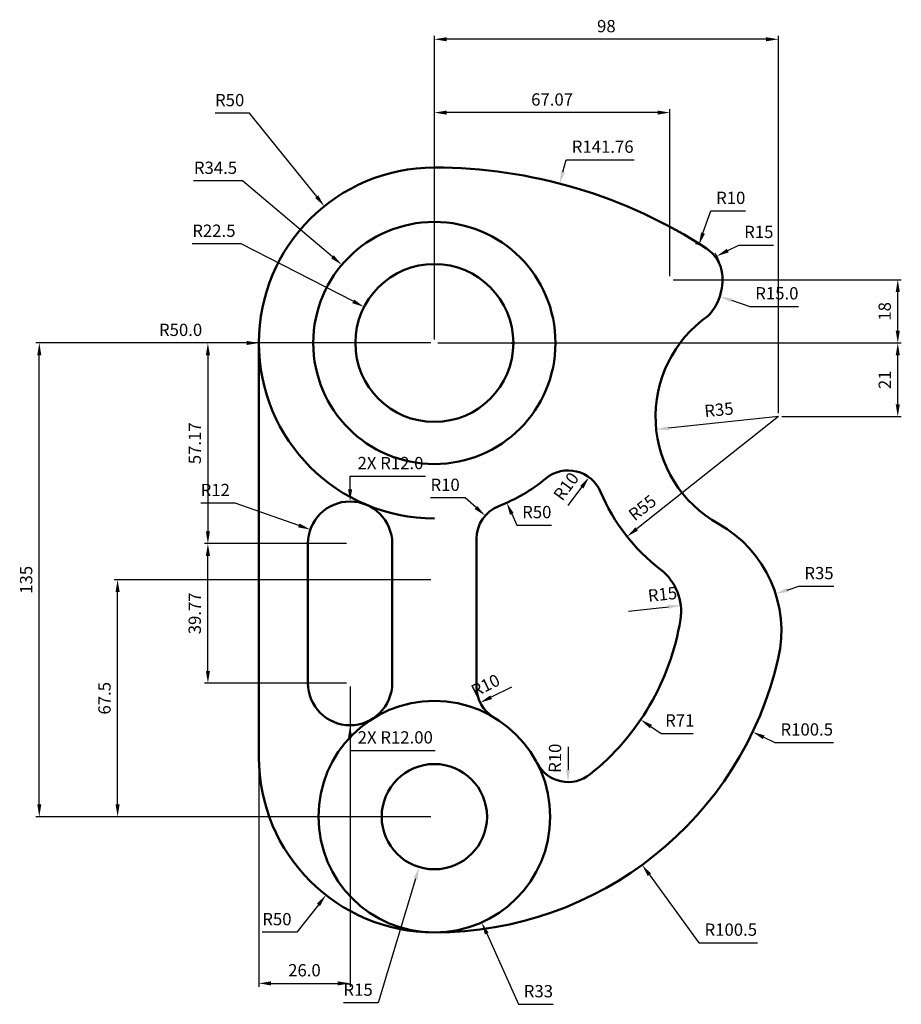
# Model space of a CAD drawing. Units: millimetres. Extents: x 220 to 471, y 51 to 332.
import ezdxf

# ---------------------------------------------------------------- set-up
doc = ezdxf.new("R2010")
doc.units = ezdxf.units.MM
doc.layers.add('M-DIMS', color=3, linetype='Continuous', lineweight=25)
doc.layers.add('M-OUTL', color=7, linetype='Continuous', lineweight=50)
doc.styles.get("Standard").update_dxf_attribs({"font": 'arial.ttf'})
doc.dimstyles.new('AM_ISO$0', dxfattribs={"dimtxt": 3.5, "dimasz": 3.5, "dimexe": 1, "dimexo": 1, "dimgap": 1.5, "dimtad": 1, "dimdsep": 46, "dimtxsty": 'Standard', "dimcen": 0, "dimclrd": 256, "dimclre": 256, "dimadec": 0, "dimazin": 2, "dimtp": 0.1, "dimtm": 0.1, "dimtfac": 0.71, "dimtmove": 0, "dimatfit": 3, "dimfxl": 1, "dimlwd": -1, "dimlwe": -1, "dimarcsym": 1})
doc.dimstyles.new('AM_ISO$4', dxfattribs={"dimtxt": 3.5, "dimasz": 3.5, "dimexe": 1, "dimexo": 1, "dimgap": 1.5, "dimtad": 1, "dimtoh": 1, "dimdsep": 46, "dimtxsty": 'Standard', "dimcen": 0, "dimclrd": 256, "dimclre": 256, "dimadec": 0, "dimazin": 2, "dimtp": 0.1, "dimtm": 0.1, "dimtfac": 0.71, "dimtofl": 0, "dimtmove": 0, "dimatfit": 0, "dimfxl": 1, "dimlwd": -1, "dimlwe": -1, "dimarcsym": 1})

# ---------------------------------------------------------------- blocks, each defined once
blk = doc.blocks.new('*D2')
at = {"layer": 'Defpoints', "color": 0, "transparency": 16777216}
for p in [(225.55, 239.4), (338.07, 239.4), (338.07, 104.4)]:
    blk.add_point(p, dxfattribs=at)
at = {"layer": 'M-DIMS', "color": 0, "linetype": 'ByBlock', "transparency": 16777216}
for p, q in [((337.07, 239.4), (224.55, 239.4)), ((225.55, 107.9), (225.55, 235.9)), ((337.07, 104.4), (224.55, 104.4))]:
    blk.add_line(p, q, dxfattribs=at)
at = {"layer": 'M-DIMS', "color": 0, "transparency": 16777216}
for points in [[(224.97, 235.9), (226.13, 235.9), (225.55, 239.4)], [(224.97, 107.9), (226.13, 107.9), (225.55, 104.4)]]:
    blk.add_solid(points, dxfattribs=at)
at = {"layer": 'M-DIMS', "color": 0, "transparency": 16777216, "insert": (222.26, 171.9), "char_height": 3.5, "attachment_point": 5, "rotation": 90}
blk.add_mtext('135', dxfattribs=at)
blk = doc.blocks.new('*D3')
at = {"layer": 'Defpoints', "color": 0, "transparency": 16777216}
for p in [(405.14, 257.4), (470.07, 257.4), (338.07, 239.4)]:
    blk.add_point(p, dxfattribs=at)
at = {"layer": 'M-DIMS', "color": 0, "linetype": 'ByBlock', "transparency": 16777216}
for p, q in [((406.14, 257.4), (471.07, 257.4)), ((470.07, 242.9), (470.07, 253.9)), ((339.07, 239.4), (471.07, 239.4))]:
    blk.add_line(p, q, dxfattribs=at)
at = {"layer": 'M-DIMS', "color": 0, "transparency": 16777216}
for points in [[(469.49, 253.9), (470.66, 253.9), (470.07, 257.4)], [(469.49, 242.9), (470.66, 242.9), (470.07, 239.4)]]:
    blk.add_solid(points, dxfattribs=at)
at = {"layer": 'M-DIMS', "color": 0, "transparency": 16777216, "insert": (466.79, 248.4), "char_height": 3.5, "attachment_point": 5, "rotation": 90}
blk.add_mtext('18', dxfattribs=at)
blk = doc.blocks.new('*D4')
at = {"layer": 'Defpoints', "color": 0, "transparency": 16777216}
for p in [(338.07, 239.4), (470.07, 239.4), (436.07, 218.4)]:
    blk.add_point(p, dxfattribs=at)
at = {"layer": 'M-DIMS', "color": 0, "linetype": 'ByBlock', "transparency": 16777216}
for p, q in [((339.07, 239.4), (471.07, 239.4)), ((470.07, 221.9), (470.07, 235.9)), ((437.07, 218.4), (471.07, 218.4))]:
    blk.add_line(p, q, dxfattribs=at)
at = {"layer": 'M-DIMS', "color": 0, "transparency": 16777216}
for points in [[(469.49, 235.9), (470.66, 235.9), (470.07, 239.4)], [(469.49, 221.9), (470.66, 221.9), (470.07, 218.4)]]:
    blk.add_solid(points, dxfattribs=at)
at = {"layer": 'M-DIMS', "color": 0, "transparency": 16777216, "insert": (466.82, 228.9), "char_height": 3.5, "attachment_point": 5, "rotation": 90}
blk.add_mtext('21', dxfattribs=at)
blk = doc.blocks.new('*D5')
at = {"layer": 'Defpoints', "color": 0, "transparency": 16777216}
for p in [(247.85, 171.9), (338.07, 171.9), (338.07, 104.4)]:
    blk.add_point(p, dxfattribs=at)
at = {"layer": 'M-DIMS', "color": 0, "linetype": 'ByBlock', "transparency": 16777216}
for p, q in [((337.07, 171.9), (246.85, 171.9)), ((247.85, 107.9), (247.85, 168.4)), ((337.07, 104.4), (246.85, 104.4))]:
    blk.add_line(p, q, dxfattribs=at)
at = {"layer": 'M-DIMS', "color": 0, "transparency": 16777216}
for points in [[(247.27, 168.4), (248.44, 168.4), (247.85, 171.9)], [(247.27, 107.9), (248.44, 107.9), (247.85, 104.4)]]:
    blk.add_solid(points, dxfattribs=at)
at = {"layer": 'M-DIMS', "color": 0, "transparency": 16777216, "insert": (244.57, 138.15), "char_height": 3.5, "attachment_point": 5, "rotation": 90}
blk.add_mtext('67.5', dxfattribs=at)
blk = doc.blocks.new('*D6')
at = {"layer": 'Defpoints', "color": 0, "transparency": 16777216}
for p in [(338.07, 305.05), (405.14, 257.4), (338.07, 239.4)]:
    blk.add_point(p, dxfattribs=at)
at = {"layer": 'M-DIMS', "color": 0, "linetype": 'ByBlock', "transparency": 16777216}
for p, q in [((338.07, 240.4), (338.07, 306.05)), ((405.14, 258.4), (405.14, 306.05)), ((401.64, 305.05), (341.57, 305.05))]:
    blk.add_line(p, q, dxfattribs=at)
at = {"layer": 'M-DIMS', "color": 0, "transparency": 16777216}
for points in [[(341.57, 305.63), (341.57, 304.46), (338.07, 305.05)], [(401.64, 305.63), (401.64, 304.46), (405.14, 305.05)]]:
    blk.add_solid(points, dxfattribs=at)
at = {"layer": 'M-DIMS', "color": 0, "transparency": 16777216, "insert": (371.61, 308.33), "char_height": 3.5, "attachment_point": 5}
blk.add_mtext('67.07', dxfattribs=at)
blk = doc.blocks.new('*D7')
at = {"layer": 'Defpoints', "color": 0, "transparency": 16777216}
for p in [(338.07, 325.94), (338.07, 239.4), (436.07, 218.4)]:
    blk.add_point(p, dxfattribs=at)
at = {"layer": 'M-DIMS', "color": 0, "linetype": 'ByBlock', "transparency": 16777216}
for p, q in [((338.07, 240.4), (338.07, 326.94)), ((432.57, 325.94), (341.57, 325.94)), ((436.07, 219.4), (436.07, 326.94))]:
    blk.add_line(p, q, dxfattribs=at)
at = {"layer": 'M-DIMS', "color": 0, "transparency": 16777216}
for points in [[(341.57, 326.52), (341.57, 325.36), (338.07, 325.94)], [(432.57, 326.52), (432.57, 325.36), (436.07, 325.94)]]:
    blk.add_solid(points, dxfattribs=at)
at = {"layer": 'M-DIMS', "color": 0, "transparency": 16777216, "insert": (387.07, 329.23), "char_height": 3.5, "attachment_point": 5}
blk.add_mtext('98', dxfattribs=at)
blk = doc.blocks.new('*D8')
at = {"layer": 'Defpoints', "color": 0, "transparency": 16777216}
for p in [(373.81, 284.82), (338.07, 147.64)]:
    blk.add_point(p, dxfattribs=at)
at = {"layer": 'M-DIMS', "color": 0, "linetype": 'ByBlock', "transparency": 16777216}
for p, q in [((374.69, 288.21), (375.58, 291.59)), ((375.58, 291.59), (394.95, 291.59))]:
    blk.add_line(p, q, dxfattribs=at)
at = {"layer": 'M-DIMS', "color": 0, "transparency": 16777216}
blk.add_solid([(374.13, 288.35), (375.26, 288.06), (373.81, 284.82)], dxfattribs=at)
at = {"layer": 'M-DIMS', "color": 0, "transparency": 16777216, "insert": (386.02, 294.88), "char_height": 3.5, "attachment_point": 5}
blk.add_mtext('R141.76', dxfattribs=at)
blk = doc.blocks.new('*D9')
at = {"layer": 'Defpoints', "color": 0, "transparency": 16777216}
for p in [(413.43, 267.39), (410.11, 257.96)]:
    blk.add_point(p, dxfattribs=at)
at = {"layer": 'M-DIMS', "color": 0, "linetype": 'ByBlock', "transparency": 16777216}
for p, q in [((414.59, 270.7), (416.81, 277.01)), ((416.81, 277.01), (426.67, 277.01))]:
    blk.add_line(p, q, dxfattribs=at)
blk.add_arc((410.11, 257.96), 10, 62.5869, 76.3385, dxfattribs=at)
at = {"layer": 'M-DIMS', "color": 0, "transparency": 16777216}
blk.add_solid([(414.04, 270.89), (415.14, 270.5), (413.43, 267.39)], dxfattribs=at)
at = {"layer": 'M-DIMS', "color": 0, "transparency": 16777216, "insert": (422.49, 280.3), "char_height": 3.5, "attachment_point": 5}
blk.add_mtext('R10', dxfattribs=at)
blk = doc.blocks.new('*D10')
at = {"layer": 'Defpoints', "color": 0, "transparency": 16777216}
for p in [(418.53, 264.15), (405.14, 257.4)]:
    blk.add_point(p, dxfattribs=at)
at = {"layer": 'M-DIMS', "color": 0, "linetype": 'ByBlock', "transparency": 16777216}
for p, q in [((421.66, 265.73), (424.78, 267.31)), ((424.78, 267.31), (434.67, 267.31))]:
    blk.add_line(p, q, dxfattribs=at)
blk.add_arc((405.14, 257.4), 15, 10.2983, 30.5884, dxfattribs=at)
at = {"layer": 'M-DIMS', "color": 0, "transparency": 16777216}
blk.add_solid([(421.4, 266.25), (421.92, 265.21), (418.53, 264.15)], dxfattribs=at)
at = {"layer": 'M-DIMS', "color": 0, "transparency": 16777216, "insert": (430.48, 270.59), "char_height": 3.5, "attachment_point": 5}
blk.add_mtext('R15', dxfattribs=at)
blk = doc.blocks.new('*D11')
at = {"layer": 'Defpoints', "color": 0, "transparency": 16777216}
for p in [(352.57, 190.18), (360.07, 183.58)]:
    blk.add_point(p, dxfattribs=at)
at = {"layer": 'M-DIMS', "color": 0, "linetype": 'ByBlock', "transparency": 16777216}
for p, q in [((346.81, 195.25), (336.96, 195.25)), ((349.94, 192.5), (346.81, 195.25))]:
    blk.add_line(p, q, dxfattribs=at)
at = {"layer": 'M-DIMS', "color": 0, "transparency": 16777216}
blk.add_solid([(350.32, 192.93), (349.55, 192.06), (352.57, 190.18)], dxfattribs=at)
at = {"layer": 'M-DIMS', "color": 0, "transparency": 16777216, "insert": (341.14, 198.53), "char_height": 3.5, "attachment_point": 5}
blk.add_mtext('R10', dxfattribs=at)
blk = doc.blocks.new('*D12')
at = {"layer": 'Defpoints', "color": 0, "transparency": 16777216}
for p in [(360.07, 141.34), (351.12, 136.89)]:
    blk.add_point(p, dxfattribs=at)
at = {"layer": 'M-DIMS', "color": 0, "linetype": 'ByBlock', "transparency": 16777216}
blk.add_line((360.07, 141.34), (354.25, 138.45), dxfattribs=at)
at = {"layer": 'M-DIMS', "color": 0, "transparency": 16777216}
blk.add_solid([(353.99, 138.97), (354.51, 137.93), (351.12, 136.89)], dxfattribs=at)
at = {"layer": 'M-DIMS', "color": 0, "transparency": 16777216, "insert": (352.83, 141.42), "char_height": 3.5, "attachment_point": 5, "rotation": 26.4394}
blk.add_mtext('R10', dxfattribs=at)
blk = doc.blocks.new('*D13')
at = {"layer": 'Defpoints', "color": 0, "transparency": 16777216}
for p in [(376.2, 124.28), (376.14, 114.28)]:
    blk.add_point(p, dxfattribs=at)
at = {"layer": 'M-DIMS', "color": 0, "linetype": 'ByBlock', "transparency": 16777216}
blk.add_line((376.2, 124.28), (376.16, 117.78), dxfattribs=at)
at = {"layer": 'M-DIMS', "color": 0, "transparency": 16777216}
blk.add_solid([(375.58, 117.79), (376.74, 117.78), (376.14, 114.28)], dxfattribs=at)
at = {"layer": 'M-DIMS', "color": 0, "transparency": 16777216, "insert": (372.89, 121.05), "char_height": 3.5, "attachment_point": 5, "rotation": 89.6408}
blk.add_mtext('R10', dxfattribs=at)
blk = doc.blocks.new('*D14')
at = {"layer": 'Defpoints', "color": 0, "transparency": 16777216}
for p in [(338.07, 171.9), (396.84, 132.06)]:
    blk.add_point(p, dxfattribs=at)
at = {"layer": 'M-DIMS', "color": 0, "linetype": 'ByBlock', "transparency": 16777216}
for p, q in [((399.74, 130.09), (402.63, 128.13)), ((402.63, 128.13), (411.82, 128.13))]:
    blk.add_line(p, q, dxfattribs=at)
at = {"layer": 'M-DIMS', "color": 0, "transparency": 16777216}
blk.add_solid([(400.06, 130.57), (399.41, 129.61), (396.84, 132.06)], dxfattribs=at)
at = {"layer": 'M-DIMS', "color": 0, "transparency": 16777216, "insert": (407.98, 131.38), "char_height": 3.5, "attachment_point": 5}
blk.add_mtext('R71', dxfattribs=at)
blk = doc.blocks.new('*D15')
at = {"layer": 'Defpoints', "color": 0, "transparency": 16777216}
for p in [(393.35, 162.95), (408.26, 164.6)]:
    blk.add_point(p, dxfattribs=at)
at = {"layer": 'M-DIMS', "color": 0, "linetype": 'ByBlock', "transparency": 16777216}
blk.add_line((393.35, 162.95), (404.78, 164.22), dxfattribs=at)
at = {"layer": 'M-DIMS', "color": 0, "transparency": 16777216}
blk.add_solid([(404.72, 164.8), (404.85, 163.64), (408.26, 164.6)], dxfattribs=at)
at = {"layer": 'M-DIMS', "color": 0, "transparency": 16777216, "insert": (403.09, 167.33), "char_height": 3.5, "attachment_point": 5, "rotation": 6.3399}
blk.add_mtext('R15', dxfattribs=at)
blk = doc.blocks.new('*D16')
at = {"layer": 'Defpoints', "color": 0, "transparency": 16777216}
for p in [(436.07, 218.4), (392.97, 184.23)]:
    blk.add_point(p, dxfattribs=at)
at = {"layer": 'M-DIMS', "color": 0, "linetype": 'ByBlock', "transparency": 16777216}
blk.add_line((436.07, 218.4), (395.72, 186.41), dxfattribs=at)
at = {"layer": 'M-DIMS', "color": 0, "transparency": 16777216}
blk.add_solid([(395.35, 186.86), (396.08, 185.95), (392.97, 184.23)], dxfattribs=at)
at = {"layer": 'M-DIMS', "color": 0, "transparency": 16777216, "insert": (397.6, 192.09), "char_height": 3.5, "attachment_point": 5, "rotation": 38.405}
blk.add_mtext('R55', dxfattribs=at)
blk = doc.blocks.new('*D17')
at = {"layer": 'Defpoints', "color": 0, "transparency": 16777216}
for p in [(382.15, 201.12), (376.21, 193.08)]:
    blk.add_point(p, dxfattribs=at)
at = {"layer": 'M-DIMS', "color": 0, "linetype": 'ByBlock', "transparency": 16777216}
blk.add_line((376.21, 193.08), (380.07, 198.3), dxfattribs=at)
at = {"layer": 'M-DIMS', "color": 0, "transparency": 16777216}
blk.add_solid([(379.6, 198.65), (380.54, 197.96), (382.15, 201.12)], dxfattribs=at)
at = {"layer": 'M-DIMS', "color": 0, "transparency": 16777216, "insert": (375.95, 198.26), "char_height": 3.5, "attachment_point": 5, "rotation": 53.5261}
blk.add_mtext('R10', dxfattribs=at)
blk = doc.blocks.new('*D18')
at = {"layer": 'Defpoints', "color": 0, "transparency": 16777216}
for p in [(338.07, 239.4), (358.69, 193.84)]:
    blk.add_point(p, dxfattribs=at)
at = {"layer": 'M-DIMS', "color": 0, "linetype": 'ByBlock', "transparency": 16777216}
for p, q in [((360.13, 190.66), (361.57, 187.47)), ((361.57, 187.47), (371.42, 187.47))]:
    blk.add_line(p, q, dxfattribs=at)
at = {"layer": 'M-DIMS', "color": 0, "transparency": 16777216}
blk.add_solid([(360.66, 190.9), (359.6, 190.42), (358.69, 193.84)], dxfattribs=at)
at = {"layer": 'M-DIMS', "color": 0, "transparency": 16777216, "insert": (367.25, 190.75), "char_height": 3.5, "attachment_point": 5}
blk.add_mtext('R50', dxfattribs=at)
blk = doc.blocks.new('*D19')
at = {"layer": 'Defpoints', "color": 0, "transparency": 16777216}
for p in [(338.07, 171.9), (428.74, 128.54)]:
    blk.add_point(p, dxfattribs=at)
at = {"layer": 'M-DIMS', "color": 0, "linetype": 'ByBlock', "transparency": 16777216}
for p, q in [((431.9, 127.03), (435.05, 125.52)), ((435.05, 125.52), (451.74, 125.52))]:
    blk.add_line(p, q, dxfattribs=at)
at = {"layer": 'M-DIMS', "color": 0, "transparency": 16777216}
blk.add_solid([(432.15, 127.56), (431.65, 126.5), (428.74, 128.54)], dxfattribs=at)
at = {"layer": 'M-DIMS', "color": 0, "transparency": 16777216, "insert": (444.15, 128.81), "char_height": 3.5, "attachment_point": 5}
blk.add_mtext('R100.5', dxfattribs=at)
blk = doc.blocks.new('*D20')
at = {"layer": 'Defpoints', "color": 0, "transparency": 16777216}
for p in [(435.27, 167.94), (401.92, 157.29)]:
    blk.add_point(p, dxfattribs=at)
at = {"layer": 'M-DIMS', "color": 0, "linetype": 'ByBlock', "transparency": 16777216}
for p, q in [((438.6, 169), (441.93, 170.07)), ((441.93, 170.07), (451.82, 170.07))]:
    blk.add_line(p, q, dxfattribs=at)
at = {"layer": 'M-DIMS', "color": 0, "transparency": 16777216}
blk.add_solid([(438.42, 169.56), (438.78, 168.45), (435.27, 167.94)], dxfattribs=at)
at = {"layer": 'M-DIMS', "color": 0, "transparency": 16777216, "insert": (447.63, 173.36), "char_height": 3.5, "attachment_point": 5}
blk.add_mtext('R35', dxfattribs=at)
blk = doc.blocks.new('*D21')
at = {"layer": 'Defpoints', "color": 0, "transparency": 16777216}
for p in [(436.07, 218.4), (401.26, 214.75)]:
    blk.add_point(p, dxfattribs=at)
at = {"layer": 'M-DIMS', "color": 0, "linetype": 'ByBlock', "transparency": 16777216}
blk.add_line((436.07, 218.4), (404.74, 215.12), dxfattribs=at)
at = {"layer": 'M-DIMS', "color": 0, "transparency": 16777216}
blk.add_solid([(404.68, 215.7), (404.8, 214.54), (401.26, 214.75)], dxfattribs=at)
at = {"layer": 'M-DIMS', "color": 0, "transparency": 16777216, "insert": (419.17, 219.93), "char_height": 3.5, "attachment_point": 5, "rotation": 5.979}
blk.add_mtext('R35', dxfattribs=at)
blk = doc.blocks.new('*D22')
at = {"layer": 'Defpoints', "color": 0, "transparency": 16777216}
for p in [(338.07, 121.4), (307.21, 82.06)]:
    blk.add_point(p, dxfattribs=at)
at = {"layer": 'M-DIMS', "color": 0, "linetype": 'ByBlock', "transparency": 16777216}
for p, q in [((305.05, 79.3), (298.91, 71.46)), ((298.91, 71.46), (289.05, 71.46))]:
    blk.add_line(p, q, dxfattribs=at)
at = {"layer": 'M-DIMS', "color": 0, "transparency": 16777216}
blk.add_solid([(304.6, 79.66), (305.51, 78.94), (307.21, 82.06)], dxfattribs=at)
at = {"layer": 'M-DIMS', "color": 0, "transparency": 16777216, "insert": (293.23, 74.75), "char_height": 3.5, "attachment_point": 5}
blk.add_mtext('R50', dxfattribs=at)
blk = doc.blocks.new('*D23')
at = {"layer": 'Defpoints', "color": 0, "transparency": 16777216}
for p in [(338.07, 171.9), (397.25, 90.67)]:
    blk.add_point(p, dxfattribs=at)
at = {"layer": 'M-DIMS', "color": 0, "linetype": 'ByBlock', "transparency": 16777216}
for p, q in [((399.31, 87.84), (413.41, 68.47)), ((413.41, 68.47), (430.1, 68.47))]:
    blk.add_line(p, q, dxfattribs=at)
at = {"layer": 'M-DIMS', "color": 0, "transparency": 16777216}
blk.add_solid([(399.78, 88.18), (398.84, 87.49), (397.25, 90.67)], dxfattribs=at)
at = {"layer": 'M-DIMS', "color": 0, "transparency": 16777216, "insert": (422.51, 71.76), "char_height": 3.5, "attachment_point": 5}
blk.add_mtext('R100.5', dxfattribs=at)
blk = doc.blocks.new('*D24')
at = {"layer": 'Defpoints', "color": 0, "transparency": 16777216}
for p in [(338.07, 104.4), (351.57, 74.28)]:
    blk.add_point(p, dxfattribs=at)
at = {"layer": 'M-DIMS', "color": 0, "linetype": 'ByBlock', "transparency": 16777216}
for p, q in [((353, 71.09), (362.03, 50.93)), ((362.03, 50.93), (371.9, 50.93))]:
    blk.add_line(p, q, dxfattribs=at)
at = {"layer": 'M-DIMS', "color": 0, "transparency": 16777216}
blk.add_solid([(353.53, 71.33), (352.47, 70.85), (351.57, 74.28)], dxfattribs=at)
at = {"layer": 'M-DIMS', "color": 0, "transparency": 16777216, "insert": (367.71, 54.22), "char_height": 3.5, "attachment_point": 5}
blk.add_mtext('R33', dxfattribs=at)
blk = doc.blocks.new('*D25')
at = {"layer": 'Defpoints', "color": 0, "transparency": 16777216}
for p in [(338.07, 104.4), (333.73, 90.04)]:
    blk.add_point(p, dxfattribs=at)
at = {"layer": 'M-DIMS', "color": 0, "linetype": 'ByBlock', "transparency": 16777216}
for p, q in [((332.72, 86.69), (322.04, 51.36)), ((322.04, 51.36), (312.15, 51.36))]:
    blk.add_line(p, q, dxfattribs=at)
at = {"layer": 'M-DIMS', "color": 0, "transparency": 16777216}
blk.add_solid([(332.16, 86.86), (333.28, 86.52), (333.73, 90.04)], dxfattribs=at)
at = {"layer": 'M-DIMS', "color": 0, "transparency": 16777216, "insert": (316.35, 54.65), "char_height": 3.5, "attachment_point": 5}
blk.add_mtext('R15', dxfattribs=at)
blk = doc.blocks.new('*D26')
at = {"layer": 'Defpoints', "color": 0, "transparency": 16777216}
for p in [(302.76, 186.23), (314.07, 182.23)]:
    blk.add_point(p, dxfattribs=at)
at = {"layer": 'M-DIMS', "color": 0, "linetype": 'ByBlock', "transparency": 16777216}
for p, q in [((281.34, 193.79), (271.52, 193.79)), ((299.46, 187.39), (281.34, 193.79))]:
    blk.add_line(p, q, dxfattribs=at)
at = {"layer": 'M-DIMS', "color": 0, "transparency": 16777216}
blk.add_solid([(299.65, 187.94), (299.26, 186.84), (302.76, 186.23)], dxfattribs=at)
at = {"layer": 'M-DIMS', "color": 0, "transparency": 16777216, "insert": (275.68, 197.05), "char_height": 3.5, "attachment_point": 5}
blk.add_mtext('R12', dxfattribs=at)
blk = doc.blocks.new('*D27')
at = {"layer": 'Defpoints', "color": 0, "transparency": 16777216}
for p in [(306.75, 278.37), (338.07, 239.4)]:
    blk.add_point(p, dxfattribs=at)
at = {"layer": 'M-DIMS', "color": 0, "linetype": 'ByBlock', "transparency": 16777216}
for p, q in [((285.45, 304.87), (275.6, 304.87)), ((304.56, 281.1), (285.45, 304.87))]:
    blk.add_line(p, q, dxfattribs=at)
at = {"layer": 'M-DIMS', "color": 0, "transparency": 16777216}
blk.add_solid([(305.01, 281.46), (304.1, 280.73), (306.75, 278.37)], dxfattribs=at)
at = {"layer": 'M-DIMS', "color": 0, "transparency": 16777216, "insert": (279.77, 308.16), "char_height": 3.5, "attachment_point": 5}
blk.add_mtext('R50', dxfattribs=at)
blk = doc.blocks.new('*D28')
at = {"layer": 'Defpoints', "color": 0, "transparency": 16777216}
for p in [(311.73, 261.68), (338.07, 239.4)]:
    blk.add_point(p, dxfattribs=at)
at = {"layer": 'M-DIMS', "color": 0, "linetype": 'ByBlock', "transparency": 16777216}
for p, q in [((283.47, 285.59), (269.5, 285.59)), ((309.06, 263.94), (283.47, 285.59))]:
    blk.add_line(p, q, dxfattribs=at)
at = {"layer": 'M-DIMS', "color": 0, "transparency": 16777216}
blk.add_solid([(309.44, 264.38), (308.68, 263.49), (311.73, 261.68)], dxfattribs=at)
at = {"layer": 'M-DIMS', "color": 0, "transparency": 16777216, "insert": (275.73, 288.87), "char_height": 3.5, "attachment_point": 5}
blk.add_mtext('R34.5', dxfattribs=at)
blk = doc.blocks.new('*D29')
at = {"layer": 'Defpoints', "color": 0, "transparency": 16777216}
for p in [(318.05, 249.67), (338.07, 239.4)]:
    blk.add_point(p, dxfattribs=at)
at = {"layer": 'M-DIMS', "color": 0, "linetype": 'ByBlock', "transparency": 16777216}
for p, q in [((283.02, 267.65), (269.05, 267.65)), ((314.94, 251.27), (283.02, 267.65))]:
    blk.add_line(p, q, dxfattribs=at)
at = {"layer": 'M-DIMS', "color": 0, "transparency": 16777216}
blk.add_solid([(315.21, 251.79), (314.67, 250.75), (318.05, 249.67)], dxfattribs=at)
at = {"layer": 'M-DIMS', "color": 0, "transparency": 16777216, "insert": (275.28, 270.93), "char_height": 3.5, "attachment_point": 5}
blk.add_mtext('R22.5', dxfattribs=at)
blk = doc.blocks.new('*D30')
at = {"layer": 'Defpoints', "color": 0, "transparency": 16777216}
for p in [(314.07, 142.46), (288.07, 121.4), (314.07, 56.9)]:
    blk.add_point(p, dxfattribs=at)
at = {"layer": 'M-DIMS', "linetype": 'ByBlock', "transparency": 16777216}
for p, q in [((314.07, 141.46), (314.07, 55.9)), ((288.07, 120.4), (288.07, 55.9)), ((291.57, 56.9), (310.57, 56.9))]:
    blk.add_line(p, q, dxfattribs=at)
at = {"layer": 'M-DIMS', "transparency": 16777216}
for points in [[(291.57, 57.48), (291.57, 56.31), (288.07, 56.9)], [(310.57, 57.48), (310.57, 56.31), (314.07, 56.9)]]:
    blk.add_solid(points, dxfattribs=at)
at = {"layer": 'M-DIMS', "color": 0, "transparency": 16777216, "insert": (301.07, 60.19), "char_height": 3.5, "attachment_point": 5}
blk.add_mtext('26.0', dxfattribs=at)
blk = doc.blocks.new('*D31')
at = {"layer": 'Defpoints', "color": 0, "transparency": 16777216}
for p in [(273.57, 182.23), (314.07, 182.23), (314.07, 142.46)]:
    blk.add_point(p, dxfattribs=at)
at = {"layer": 'M-DIMS', "linetype": 'ByBlock', "transparency": 16777216}
for p, q in [((313.07, 182.23), (272.57, 182.23)), ((273.57, 145.96), (273.57, 178.73)), ((313.07, 142.46), (272.57, 142.46))]:
    blk.add_line(p, q, dxfattribs=at)
at = {"layer": 'M-DIMS', "transparency": 16777216}
for points in [[(272.99, 178.73), (274.16, 178.73), (273.57, 182.23)], [(272.99, 145.96), (274.16, 145.96), (273.57, 142.46)]]:
    blk.add_solid(points, dxfattribs=at)
at = {"layer": 'M-DIMS', "color": 0, "transparency": 16777216, "insert": (270.28, 162.35), "char_height": 3.5, "attachment_point": 5, "rotation": 90}
blk.add_mtext('39.77', dxfattribs=at)
blk = doc.blocks.new('*D32')
at = {"layer": 'Defpoints', "color": 0, "transparency": 16777216}
for p in [(405.14, 257.4), (419.37, 252.66)]:
    blk.add_point(p, dxfattribs=at)
at = {"layer": 'M-DIMS', "linetype": 'ByBlock', "transparency": 16777216}
for p, q in [((422.69, 251.55), (427.91, 249.82)), ((427.91, 249.82), (441.84, 249.82))]:
    blk.add_line(p, q, dxfattribs=at)
at = {"layer": 'M-DIMS', "transparency": 16777216}
blk.add_solid([(422.88, 252.11), (422.51, 251), (419.37, 252.66)], dxfattribs=at)
at = {"layer": 'M-DIMS', "color": 0, "transparency": 16777216, "insert": (435.63, 253.1), "char_height": 3.5, "attachment_point": 5}
blk.add_mtext('R15.0', dxfattribs=at)
blk = doc.blocks.new('*D33')
at = {"layer": 'Defpoints', "color": 0, "transparency": 16777216}
for p in [(314.07, 194.23), (314.07, 182.23)]:
    blk.add_point(p, dxfattribs=at)
at = {"layer": 'M-DIMS', "linetype": 'ByBlock', "transparency": 16777216}
for p, q in [((314.07, 197.73), (314.07, 201.43)), ((314.07, 201.43), (335.58, 201.43))]:
    blk.add_line(p, q, dxfattribs=at)
at = {"layer": 'M-DIMS', "transparency": 16777216}
blk.add_solid([(313.49, 197.73), (314.66, 197.73), (314.07, 194.23)], dxfattribs=at)
at = {"layer": 'M-DIMS', "color": 0, "transparency": 16777216, "insert": (325.58, 204.72), "char_height": 3.5, "attachment_point": 5}
blk.add_mtext('2X R12.0', dxfattribs=at)
blk = doc.blocks.new('*D34')
at = {"layer": 'Defpoints', "color": 0, "transparency": 16777216}
for p in [(338.07, 239.4), (273.57, 182.23), (314.07, 182.23)]:
    blk.add_point(p, dxfattribs=at)
at = {"layer": 'M-DIMS', "linetype": 'ByBlock', "transparency": 16777216}
for p, q in [((337.07, 239.4), (272.57, 239.4)), ((273.57, 235.9), (273.57, 185.73)), ((313.07, 182.23), (272.57, 182.23))]:
    blk.add_line(p, q, dxfattribs=at)
at = {"layer": 'M-DIMS', "transparency": 16777216}
for points in [[(272.99, 235.9), (274.16, 235.9), (273.57, 239.4)], [(272.99, 185.73), (274.16, 185.73), (273.57, 182.23)]]:
    blk.add_solid(points, dxfattribs=at)
at = {"layer": 'M-DIMS', "color": 0, "transparency": 16777216, "insert": (270.29, 210.81), "char_height": 3.5, "attachment_point": 5, "rotation": 90}
blk.add_mtext('57.17', dxfattribs=at)
blk = doc.blocks.new('*D35')
at = {"layer": 'Defpoints', "color": 0, "transparency": 16777216}
for p in [(288.07, 239.4), (338.07, 239.4)]:
    blk.add_point(p, dxfattribs=at)
at = {"layer": 'M-DIMS', "linetype": 'ByBlock', "transparency": 16777216}
blk.add_line((284.57, 239.4), (273.5, 239.4), dxfattribs=at)
at = {"layer": 'M-DIMS', "transparency": 16777216}
blk.add_solid([(284.57, 239.98), (284.57, 238.81), (288.07, 239.4)], dxfattribs=at)
at = {"layer": 'M-DIMS', "color": 0, "transparency": 16777216, "insert": (265.79, 242.68), "char_height": 3.5, "attachment_point": 5}
blk.add_mtext('R50.0', dxfattribs=at)
blk = doc.blocks.new('*D36')
at = {"layer": 'Defpoints', "color": 0, "transparency": 16777216}
for p in [(314.07, 142.46), (314.07, 130.46)]:
    blk.add_point(p, dxfattribs=at)
at = {"layer": 'M-DIMS', "linetype": 'ByBlock', "transparency": 16777216}
for p, q in [((314.07, 126.96), (314.07, 123.26)), ((314.07, 123.26), (338.3, 123.26))]:
    blk.add_line(p, q, dxfattribs=at)
at = {"layer": 'M-DIMS', "transparency": 16777216}
blk.add_solid([(314.66, 126.96), (313.49, 126.96), (314.07, 130.46)], dxfattribs=at)
at = {"layer": 'M-DIMS', "color": 0, "transparency": 16777216, "insert": (326.94, 126.55), "char_height": 3.5, "attachment_point": 5}
blk.add_mtext('2X R12.00', dxfattribs=at)

msp = doc.modelspace()

# ---------------------------------------------------------------- linework, layer by layer
at = {"layer": 'M-OUTL'}
for p, q in [((288.073, 239.398), (288.073, 121.398)), ((350.073, 141.344), (350.073, 183.577)), ((302.073, 142.464), (302.073, 182.232)), ((326.073, 142.464), (326.073, 182.232))]:
    msp.add_line(p, q, dxfattribs=at)
for centre, radius in [((338.073, 239.398), 34.5), ((338.073, 239.398), 22.5), ((338.073, 104.398), 33), ((338.073, 104.398), 15)]:
    msp.add_circle(centre, radius, dxfattribs=at)
for centre, radius, start, end in [((338.073, 239.398), 50, 90, 270), ((338.073, 147.638), 141.76, 56.85732, 90), ((410.109, 257.962), 10, 6.47854, 56.85732), ((405.141, 257.398), 15, 316.69693, 6.47854), ((436.073, 218.398), 35, 124.88047, 240.80102), ((338.073, 171.898), 71, 71.52484, 71.93479), ((376.208, 193.076), 10, 22.92755, 129.46341), ((338.073, 239.398), 50, 291.51019, 309.46341), ((436.073, 218.398), 55, 202.92755, 232.38959), ((314.073, 182.232), 12, 360, 180), ((360.073, 183.577), 10, 111.51019, 180), ((401.924, 157.293), 35, 347.11591, 60.80102), ((393.352, 162.946), 15, 350.80086, 52.38959), ((338.073, 171.898), 71, 308.68436, 350.80086), ((338.073, 171.898), 100.5, 270, 347.11591), ((314.073, 142.464), 12, 180, 360), ((360.073, 141.344), 10, 180, 239.22768), ((338.073, 121.398), 50, 180, 270), ((376.2, 124.281), 10, 207.54228, 308.68436)]:
    msp.add_arc(centre, radius, start, end, dxfattribs=at)

# ---------------------------------------------------------------- dimensions: what is measured, and where the dimension line sits
at = {"layer": 'M-DIMS'}
for base, p1, p2, dimstyle, override, picture, middle in [((338.073, 325.94), (436.073, 218.398), (338.073, 239.398), 'AM_ISO$0', {"dimclrd": 0, "dimclre": 0, "dimclrt": 0}, '*D7', (387.073, 329.227)), ((338.073, 305.047), (405.141, 257.398), (338.073, 239.398), 'AM_ISO$0', {"dimpost": '', "dimclrd": 0, "dimclre": 0, "dimclrt": 0}, '*D6', (371.607, 308.334)), ((314.073, 56.898), (288.073, 121.398), (314.073, 142.464), 'AM_ISO$4', {"dimdec": 1, "dimlfac": 1, "dimrnd": 0, "dimzin": 0, "dimdsep": 46, "dimlunit": 2}, '*D30', (301.073, 60.185))]:
    dim = msp.add_linear_dim(base=base, p1=p1, p2=p2, dimstyle=dimstyle, override=override, dxfattribs=at)
    dim.commit()
    dim.dimension.update_dxf_attribs({"geometry": picture, "text_midpoint": middle})
for center, mpoint, override, picture, middle in [((338.073, 239.398), (306.748, 278.369), {"dimclrd": 0, "dimclre": 0, "dimclrt": 0}, '*D27', (279.772, 304.869)), ((338.073, 147.638), (373.812, 284.819), {"dimpost": '', "dimclrd": 0, "dimclre": 0, "dimclrt": 0}, '*D8', (386.015, 291.593)), ((338.073, 239.398), (311.731, 261.678), {"dimclrd": 0, "dimclre": 0, "dimclrt": 0}, '*D28', (275.732, 285.585)), ((410.109, 257.962), (413.43, 267.395), {"dimclrd": 0, "dimclre": 0, "dimclrt": 0}, '*D9', (422.49, 277.013)), ((338.073, 239.398), (318.054, 249.67), {"dimclrd": 0, "dimclre": 0, "dimclrt": 0}, '*D29', (275.284, 267.647)), ((405.141, 257.398), (418.534, 264.154), {"dimclrd": 0, "dimclre": 0, "dimclrt": 0}, '*D10', (430.478, 267.307)), ((405.141, 257.398), (419.373, 252.66), {"dimdec": 1, "dimlfac": 1, "dimrnd": 0, "dimzin": 0, "dimdsep": 46, "dimlunit": 2}, '*D32', (435.627, 249.817)), ((338.073, 239.398), (288.073, 239.398), {"dimdec": 1, "dimlfac": 1, "dimrnd": 0, "dimzin": 0, "dimdsep": 46, "dimlunit": 2}, '*D35', (265.787, 239.398)), ((338.073, 239.398), (358.686, 193.845), {"dimclrd": 0, "dimclre": 0, "dimclrt": 0}, '*D18', (367.247, 187.467)), ((436.073, 218.398), (401.263, 214.752), {"dimclrd": 0, "dimclre": 0, "dimclrt": 0}, '*D21', (419.511, 216.663)), ((436.073, 218.398), (392.973, 184.231), {"dimclrd": 0, "dimclre": 0, "dimclrt": 0}, '*D16', (399.639, 189.516)), ((376.208, 193.076), (382.152, 201.118), {"dimclrd": 0, "dimclre": 0, "dimclrt": 0}, '*D17', (378.594, 196.304)), ((314.073, 182.232), (302.758, 186.228), {"dimclrd": 0, "dimclre": 0, "dimclrt": 0}, '*D26', (275.68, 193.791)), ((360.073, 183.577), (352.566, 190.184), {"dimclrd": 0, "dimclre": 0, "dimclrt": 0}, '*D11', (341.139, 195.247)), ((401.924, 157.293), (435.265, 167.939), {"dimclrd": 0, "dimclre": 0, "dimclrt": 0}, '*D20', (447.628, 170.068)), ((338.073, 171.898), (396.84, 132.055), {"dimclrd": 0, "dimclre": 0, "dimclrt": 0}, '*D14', (407.977, 128.127)), ((338.073, 171.898), (428.739, 128.541), {"dimclrd": 0, "dimclre": 0, "dimclrt": 0}, '*D19', (444.148, 125.521)), ((338.073, 171.898), (397.246, 90.665), {"dimclrd": 0, "dimclre": 0, "dimclrt": 0}, '*D23', (422.507, 68.47)), ((393.352, 162.946), (408.261, 164.602), {"dimclrd": 0, "dimclre": 0, "dimclrt": 0}, '*D15', (403.451, 164.068)), ((360.073, 141.344), (351.119, 136.891), {"dimclrd": 0, "dimclre": 0, "dimclrt": 0}, '*D12', (354.298, 138.472)), ((376.2, 124.281), (376.137, 114.282), {"dimclrd": 0, "dimclre": 0, "dimclrt": 0}, '*D13', (376.179, 121.031)), ((338.073, 121.398), (307.215, 82.056), {"dimclrd": 0, "dimclre": 0, "dimclrt": 0}, '*D22', (293.23, 71.464)), ((338.073, 104.398), (333.733, 90.04), {"dimclrd": 0, "dimclre": 0, "dimclrt": 0}, '*D25', (316.346, 51.361)), ((338.073, 104.398), (351.568, 74.284), {"dimclrd": 0, "dimclre": 0, "dimclrt": 0}, '*D24', (367.714, 50.933))]:
    dim = msp.add_radius_dim(center=center, mpoint=mpoint, dimstyle='AM_ISO$4', override=override, dxfattribs=at)
    dim.commit()
    dim.dimension.update_dxf_attribs({"geometry": picture, "text_midpoint": middle, "dimtype": 164})
for base, p1, p2, dimstyle, override, picture, middle in [((470.074, 257.398), (338.073, 239.398), (405.141, 257.398), 'AM_ISO$0', {"dimclrd": 0, "dimclre": 0, "dimclrt": 0}, '*D3', (466.787, 248.398)), ((225.552, 239.398), (338.073, 104.398), (338.073, 239.398), 'AM_ISO$0', {"dimpost": '', "dimclrd": 0, "dimclre": 0, "dimclrt": 0}, '*D2', (222.263, 171.898)), ((273.573, 182.232), (338.073, 239.398), (314.073, 182.232), 'AM_ISO$4', {"dimdec": 2, "dimlfac": 1, "dimrnd": 0, "dimzin": 0, "dimdsep": 46, "dimlunit": 2}, '*D34', (270.286, 210.815)), ((470.074, 239.398), (436.073, 218.398), (338.073, 239.398), 'AM_ISO$0', {"dimclrd": 0, "dimclre": 0, "dimclrt": 0}, '*D4', (466.817, 228.898)), ((273.573, 182.232), (314.073, 142.464), (314.073, 182.232), 'AM_ISO$4', {"dimdec": 2, "dimlfac": 1, "dimrnd": 0, "dimzin": 0, "dimdsep": 46, "dimlunit": 2}, '*D31', (270.285, 162.348)), ((247.854, 171.898), (338.073, 104.398), (338.073, 171.898), 'AM_ISO$0', {"dimclrd": 0, "dimclre": 0, "dimclrt": 0}, '*D5', (244.567, 138.148))]:
    dim = msp.add_linear_dim(base=base, p1=p1, p2=p2, angle=90, dimstyle=dimstyle, override=override, dxfattribs=at)
    dim.commit()
    dim.dimension.update_dxf_attribs({"geometry": picture, "text_midpoint": middle})
for center, mpoint, override, picture, middle in [((314.073, 182.232), (314.073, 194.232), {"dimdec": 1, "dimlfac": 1, "dimrnd": 0, "dimzin": 0, "dimdsep": 46, "dimlunit": 2}, '*D33', (325.578, 201.432)), ((314.073, 142.464), (314.073, 130.464), {"dimdec": 2, "dimlfac": 1, "dimrnd": 0, "dimzin": 0, "dimdsep": 46, "dimlunit": 2}, '*D36', (326.937, 123.264))]:
    dim = msp.add_radius_dim(center=center, mpoint=mpoint, text='2X <>', dimstyle='AM_ISO$4', override=override, dxfattribs=at)
    dim.commit()
    dim.dimension.update_dxf_attribs({"geometry": picture, "text_midpoint": middle, "dimtype": 164})

doc.saveas('drawing.dxf')
